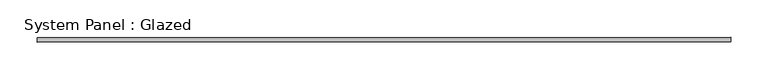
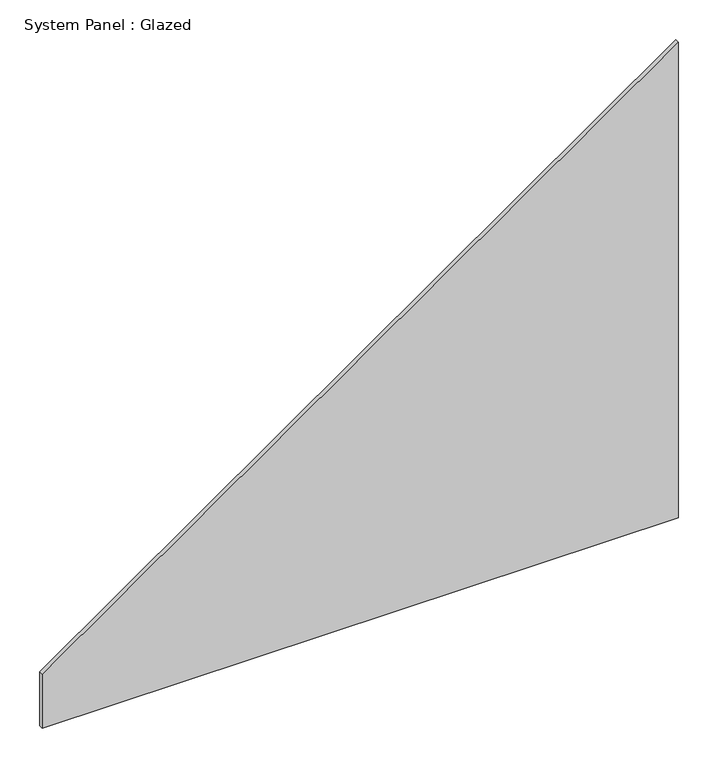
"""IFC4 building model written with IfcOpenShell, lengths in millimetres: plate geometry, System Panel : Glazed."""

from ifc_helpers import new_model, si_unit, frame, origin, place, context, project, spatial, polyline, outline, extrude, source, transform, mapped, element, save


def system_panel_glazed_28f5254f(model_context):
    return source(origin(), model_context, "Body", "SweptSolid", [
        extrude(outline(polyline([(0.0, -462.5), (0.0, 462.5), (731.0404197, 462.5), (83.3484468, -462.5), (0.0, -462.5)])), frame((0.0, 34.0, 0.0), z_axis=(0.0, 1.0, 0.0), x_axis=(0.0, 0.0, 1.0)), (0.0, 0.0, 1.0), 6.0),
    ])


if __name__ == "__main__":
    model = new_model("IFC4")
    model_context = context("Model", 3, world=origin())
    ifc_project = project(units=[si_unit("LENGTHUNIT", "METRE", prefix="MILLI")], contexts=[model_context])
    site = spatial("IfcSite", under=ifc_project)
    building = spatial("IfcBuilding", under=site)
    placement = place(None, origin())
    system_panel_glazed_shape = system_panel_glazed_28f5254f(model_context)
    element("IfcPlate", 1, ObjectType="System Panel : Glazed", at=placement, inside=building, context=model_context, shape_type="MappedRepresentation", body=[
        mapped(system_panel_glazed_shape, transform((0.0, 0.0, 0.0), x_axis=(1.0, 0.0, 0.0), y_axis=(0.0, 1.0, 0.0), z_axis=(0.0, 0.0, 1.0))),
    ])
    save(model, "model.ifc")

# Revit data of these elements
# Type "System Panel : Glazed"
#   Construction Type Id = "GSP4R"
#   Analytic Construction = "1/8 in Pilkington single glazing"
#   Visual Light Transmittance = 0.9
#   Solar Heat Gain Coefficient = 0.86
#   Heat Transfer Coefficient (U) = 6.7069 W/(m²·K)
#   Define Thermal Properties by = 1
# Element 1 (IfcPlate, "System Panel : Glazed")
#   Materials on its faces: "Default New Material(6)"
# Materials
#   "Default New Material(6)": class "Generic", colour RGB 191 25 25, transparency 0.9, Cost = 0
